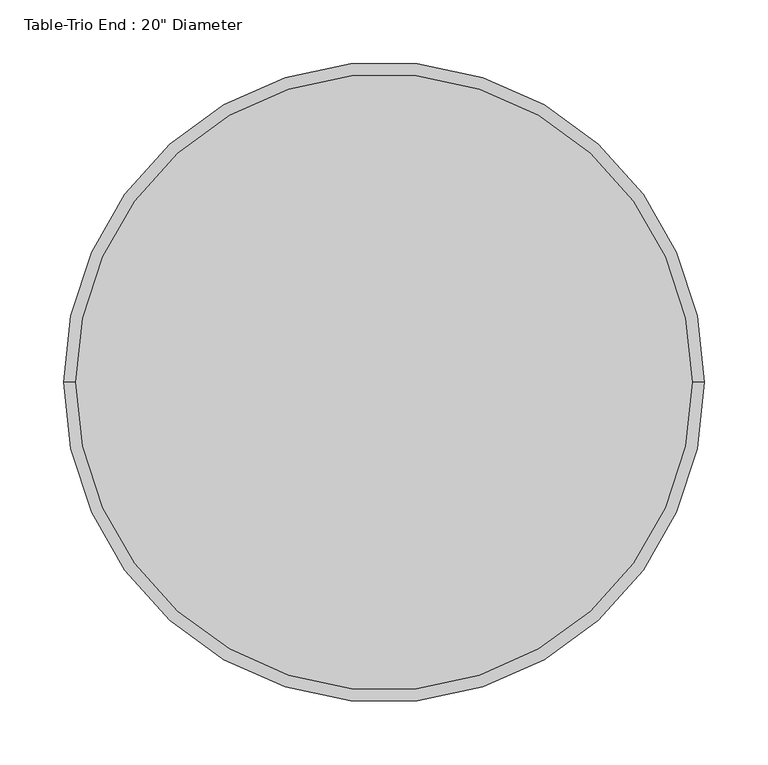
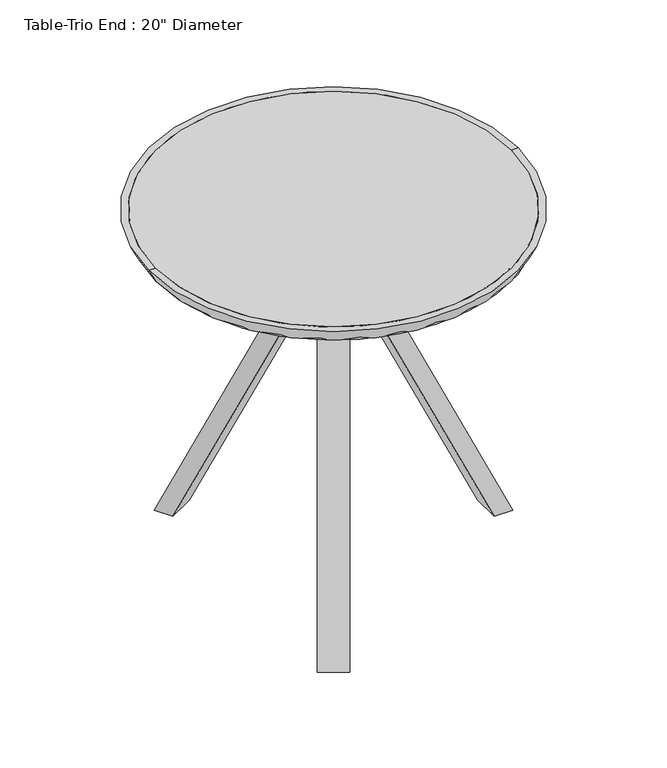
"""IFC4 building model written with IfcOpenShell, lengths in millimetres: furniture geometry."""

from ifc_helpers import new_model, si_unit, point, frame, frame_2d, origin, origin_2d, place, context, project, spatial, polyline, circle_curve, trimmed, segment, composite_curve, outline, extrude, source, transform, mapped, element, save
from ifc_brep_helpers import plane_surface, revolved_surface, advanced_brep


def furniture_9d41381f(model_context):
    return source(origin(), model_context, "Body", "SolidModel", [
        extrude(outline(composite_curve([segment(trimmed(circle_curve(origin_2d(), 241.3), [point((-241.3, 0.0))], [point((241.3, 0.0))], False, "CARTESIAN"), True, "CONTINUOUS"), segment(trimmed(circle_curve(origin_2d(), 241.3), [point((241.3, 0.0))], [point((-241.3, 0.0))], False, "CARTESIAN"), True, "CONTINUOUS")], self_intersect=False)), frame((0.0, 0.0, 482.6), z_axis=(0.0, 0.0, 1.0), x_axis=(1.0, 0.0, 0.0)), (0.0, 0.0, 1.0), 19.05),
        advanced_brep(
        [(241.3, 0.0, 482.6), (-241.3, 0.0, 482.6), (-241.3, 0.0, 501.65), (241.3, 0.0, 501.65), (250.825, 0.0, 501.65), (-250.825, 0.0, 501.65)],
        [
            (0, 1, circle_curve(frame((0.0, 0.0, 482.6), z_axis=(0.0, 0.0, -1.0), x_axis=(-1.0, 0.0, 0.0)), 241.3)),
            (1, 2),
            (2, 3, circle_curve(frame((0.0, 0.0, 501.65), z_axis=(0.0, 0.0, 1.0), x_axis=(-1.0, 0.0, 0.0)), 241.3)),
            (3, 0),
            (4, 5, circle_curve(frame((0.0, 0.0, 501.65), z_axis=(0.0, 0.0, -1.0), x_axis=(-1.0, 0.0, 0.0)), 250.825)),
            (5, 1),
            (0, 4),
            (2, 5),
            (4, 3),
            (1, 0, circle_curve(frame((0.0, 0.0, 482.6), z_axis=(0.0, 0.0, -1.0), x_axis=(1.0, 0.0, 0.0)), 241.3)),
            (3, 2, circle_curve(frame((0.0, 0.0, 501.65), z_axis=(0.0, 0.0, 1.0), x_axis=(1.0, 0.0, 0.0)), 241.3)),
            (5, 4, circle_curve(frame((0.0, 0.0, 501.65), z_axis=(0.0, 0.0, -1.0), x_axis=(1.0, 0.0, 0.0)), 250.825)),
        ],
        [
            revolved_surface(polyline([(-241.3, 0.0, 501.65), (-241.3, 0.0, 482.6)]), (0.0, 0.0, 0.0), (0.0, 0.0, 1.0)),
            revolved_surface(polyline([(-241.3, 0.0, 482.6), (-250.825, 0.0, 501.65)]), (0.0, 0.0, 0.0), (0.0, 0.0, 1.0)),
            plane_surface(frame((0.0, 0.0, 501.65), z_axis=(0.0, 0.0, 1.0), x_axis=(-1.0, 0.0, 0.0))),
            revolved_surface(polyline([(241.3, 0.0, 501.65), (241.3, 0.0, 482.6)]), (0.0, 0.0, 0.0), (0.0, 0.0, 1.0)),
            revolved_surface(polyline([(241.3, 0.0, 482.6), (250.825, 0.0, 501.65)]), (0.0, 0.0, 0.0), (0.0, 0.0, 1.0)),
            plane_surface(frame((0.0, 0.0, 501.65), z_axis=(0.0, 0.0, 1.0), x_axis=(1.0, 0.0, 0.0))),
        ],
        [
            (0, [[1, 2, 3, 4]]),
            (1, [[5, 6, -1, 7]]),
            (2, [[-3, 8, -5, 9]]),
            (3, [[10, -4, 11, -2]]),
            (4, [[12, -7, -10, -6]]),
            (5, [[-11, -9, -12, -8]]),
        ],
    ),
        extrude(outline(composite_curve([segment(polyline([(374.1964885, 32.5393466), (0.0, 207.0300348), (0.0, 232.3753669), (384.9309923, 52.8790974)]), True, "CONTINUOUS"), segment(trimmed(circle_curve(frame_2d((406.4, 98.9195329)), 50.8), [point((384.9309923, 52.8790974))], [point((457.2, 98.9195329))], True, "CARTESIAN"), True, "CONTINUOUS"), segment(polyline([(457.2, 98.9195329), (457.2, 154.8312035), (482.6, 154.8312035), (482.6, 101.6)]), True, "CONTINUOUS"), segment(trimmed(circle_curve(frame_2d((406.4, 101.6)), 76.2), [point((482.6, 101.6))], [point((374.1964885, 32.5393466))], False, "CARTESIAN"), True, "CONTINUOUS")], self_intersect=False)), frame((0.0, -19.05, 0.0), z_axis=(0.0, 1.0, 0.0), x_axis=(0.0, 0.0, 1.0)), (0.0, 0.0, 1.0), 38.1),
        extrude(outline(composite_curve([segment(trimmed(circle_curve(frame_2d((412.8801427, -76.2)), 76.2), [point((412.8801427, 0.0))], [point((481.9407961, -108.4035115))], False, "CARTESIAN"), True, "CONTINUOUS"), segment(polyline([(481.9407961, -108.4035115), (459.4443174, -156.6473658), (436.4240996, -145.9128619), (460.0533926, -95.2396796)]), True, "CONTINUOUS"), segment(trimmed(circle_curve(frame_2d((414.012957, -73.7706719)), 50.8), [point((460.0533926, -95.2396796))], [point((414.0129571, -22.9706718))], True, "CARTESIAN"), True, "CONTINUOUS"), segment(polyline([(414.0129571, -22.9706718), (-10.7114002, -22.9706719), (0.0, 0.0), (412.8801427, 0.0)]), True, "CONTINUOUS")], self_intersect=False)), frame((-120.0128014, 169.7682695, 0.0), z_axis=(0.8660254037844397, 0.4999999999999983, 0.0), x_axis=(0.2113091308703442, -0.36599815077065895, 0.9063077870366545)), (0.0, 0.0, 1.0), 38.1),
        extrude(outline(composite_curve([segment(trimmed(circle_curve(frame_2d((412.8801427, -76.2)), 76.2), [point((412.8801427, 0.0))], [point((481.9407961, -108.4035116))], False, "CARTESIAN"), True, "CONTINUOUS"), segment(polyline([(481.9407961, -108.4035116), (459.4443174, -156.6473658), (436.4240996, -145.9128619), (460.0533926, -95.2396796)]), True, "CONTINUOUS"), segment(trimmed(circle_curve(frame_2d((414.012957, -73.7706719)), 50.8), [point((460.0533926, -95.2396796))], [point((414.0129571, -22.9706718))], True, "CARTESIAN"), True, "CONTINUOUS"), segment(polyline([(414.0129571, -22.9706718), (-10.7114002, -22.9706719), (0.0, 0.0), (412.8801427, 0.0)]), True, "CONTINUOUS")], self_intersect=False)), frame((-87.0172335, -188.8182695, 0.0), z_axis=(-0.8660254037844366, 0.5000000000000038, 0.0), x_axis=(0.21130913087034656, 0.3659981507706578, 0.9063077870366544)), (0.0, 0.0, 1.0), 38.1),
        extrude(outline(composite_curve([segment(trimmed(circle_curve(origin_2d(), 31.7871474), [point((-31.7871474, 0.0))], [point((31.7871474, 0.0))], False, "CARTESIAN"), True, "CONTINUOUS"), segment(trimmed(circle_curve(origin_2d(), 31.7871474), [point((31.7871474, 0.0))], [point((-31.7871474, 0.0))], False, "CARTESIAN"), True, "CONTINUOUS")], self_intersect=False)), frame((0.0, 0.0, 381.0), z_axis=(0.0, 0.0, 1.0), x_axis=(1.0, 0.0, 0.0)), (0.0, 0.0, 1.0), 50.8),
    ])


if __name__ == "__main__":
    model = new_model("IFC4")
    model_context = context("Model", 3, world=origin())
    ifc_project = project(units=[si_unit("LENGTHUNIT", "METRE", prefix="MILLI")], contexts=[model_context])
    site = spatial("IfcSite", under=ifc_project)
    building = spatial("IfcBuilding", under=site)
    placement = place(None, origin())
    furniture_shape = furniture_9d41381f(model_context)
    element("IfcFurniture", 1, ObjectType="Table-Trio End : 20\" Diameter", at=placement, inside=building, context=model_context, shape_type="MappedRepresentation", body=[
        mapped(furniture_shape, transform((0.0, 0.0, 0.0), x_axis=(1.0, 0.0, 0.0), y_axis=(0.0, 1.0, 0.0), z_axis=(0.0, 0.0, 1.0))),
    ])
    save(model, "model.ifc")

# Revit data of these elements
# Type "Table-Trio End : 20\" Diameter"
#   Assembly Code = "E2020200"
#   Default Elevation = 0' - 6"
#   Base and Trim Material = Wood - Birch
#   Table Top Material = Laminate - Ivory,Matte
# Element 1 (IfcFurniture, "Table-Trio End : 20\" Diameter")
#   Materials on its faces: "Wood - Birch", "Laminate - Ivory,Matte"
# Materials
#   "Wood - Birch": colour RGB 230 196 162, transparency 0
#   "Laminate - Ivory,Matte": colour RGB 127 127 127, transparency 0
